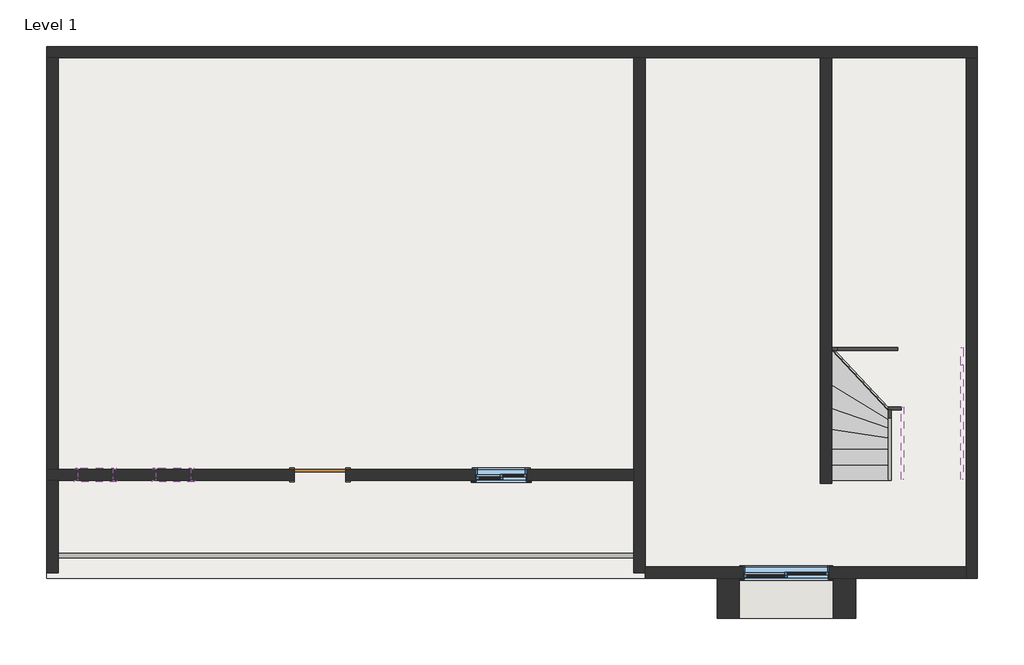
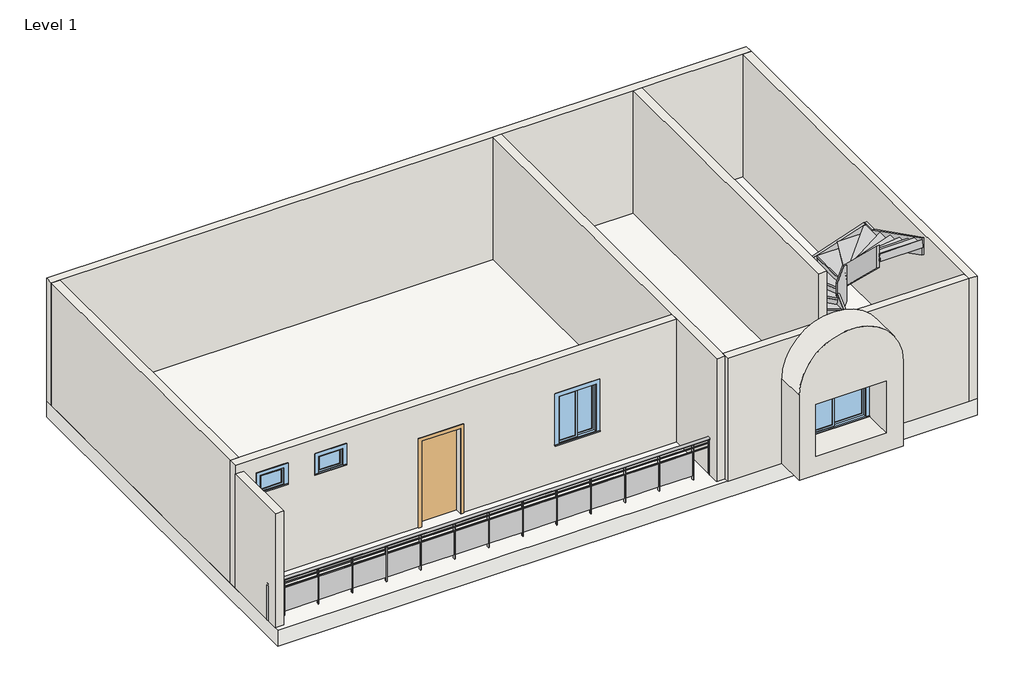
# One storey, incomplete: 9 walls, 8 members, 4 windows, 1 door, 1 railing, 1 slab, 1 stair flight.
"""IFC4 building model written with IfcOpenShell, lengths in millimetres."""

from ifc_helpers import new_model, si_unit, point, frame, origin, place, context, project, spatial, polyline, ellipse_curve, trimmed, outline, extrude, faceted_brep, transform, mapped, element, save
from ifc_brep_helpers import plane_surface, extruded_surface, advanced_brep
from components import m_single_flush_0915_x_2134mm_6a9e8738, stair_flight_50mm_tread_25mm_nosing_13mm_riser_620a4597, walls_3_walls_3_3787e265, window_242facca, window_c4d7a2b1, window_372a270f

model = new_model("IFC4")

# Units and contexts
model_context = context("Model", 3, world=origin())
ifc_project = project(units=[si_unit("LENGTHUNIT", "METRE", prefix="MILLI")], contexts=[model_context])

# Site, building, storey
site = spatial("IfcSite", under=ifc_project)
building = spatial("IfcBuilding", under=site)
storey = spatial("IfcBuildingStorey", under=building, Name="Level 1", Elevation=3048.0)

# Door
placement = place(None, origin())
m_single_flush_0915_x_2134mm_shape = m_single_flush_0915_x_2134mm_6a9e8738(model_context)
element("IfcDoor", 1, ObjectType="M_Single-Flush : 0915 x 2134mm", at=placement, inside=storey, context=model_context, shape_type="MappedRepresentation", body=[
    mapped(m_single_flush_0915_x_2134mm_shape, transform((255.2261575, -1309.9510925, 3048.0), x_axis=(1.0, 0.0, 0.0), y_axis=(0.0, 1.0, 0.0), z_axis=(0.0, 0.0, 1.0))),
])

# Members
element("IfcMember", 2, ObjectType="Stringer - 50mm Width", at=placement, inside=storey, context=model_context, shape_type="SweptSolid", body=[
    extrude(outline(polyline([(-1405.5848061, 3048.0), (-1405.5848061, 3306.6349517), (889.7143644, 4326.8592385), (889.7143644, 3889.1257613), (-1002.6491944, 3048.0), (-1405.5848061, 3048.0)])), frame((9239.7239729, 0.0, 0.0), z_axis=(1.0, 0.0, 0.0), x_axis=(0.0, 1.0, 0.0)), (0.0, 0.0, 1.0), 50.0),
])
element("IfcMember", 3, ObjectType="Stringer - 50mm Width", at=placement, inside=storey, context=model_context, shape_type="SweptSolid", body=[
    extrude(outline(polyline([(9239.7239729, 889.7143644), (9239.7239729, 939.7143644), (9388.2243256, 939.7143644), (9388.2243256, 889.7143644), (9239.7239729, 889.7143644)])), frame((0.0, 0.0, 3889.1257613), z_axis=(0.0, 0.0, 1.0), x_axis=(1.0, 0.0, 0.0)), (0.0, 0.0, 1.0), 437.7334772),
])
element("IfcMember", 4, ObjectType="Stringer - 50mm Width", at=placement, inside=storey, context=model_context, shape_type="SweptSolid", body=[
    extrude(outline(polyline([(4326.8592385, 9388.2243256), (3889.1257613, 9388.2243256), (4620.7976317, 11564.7755354), (5053.604341, 11564.7755354), (5053.604341, 11550.1195633), (4326.8592385, 9388.2243256)])), frame((0.0, 889.7143644, 0.0), z_axis=(0.0, 1.0, 0.0), x_axis=(0.0, 0.0, 1.0)), (0.0, 0.0, 1.0), 50.0),
])
element("IfcMember", 5, ObjectType="Stringer - 50mm Width", at=placement, inside=storey, context=model_context, shape_type="SweptSolid", body=[
    extrude(outline(polyline([(11564.7755354, 939.7143644), (11614.7755354, 939.7143644), (11614.7755354, 631.1318326), (11564.7755354, 631.1318326), (11564.7755354, 939.7143644)])), frame((0.0, 0.0, 4631.6082668), z_axis=(0.0, 0.0, 1.0), x_axis=(1.0, 0.0, 0.0)), (0.0, 0.0, 1.0), 421.9960743),
])
element("IfcMember", 6, ObjectType="Stringer - 50mm Width", at=placement, inside=storey, context=model_context, shape_type="SweptSolid", body=[
    extrude(outline(polyline([(631.1318326, 5053.604341), (631.1318326, 4631.6082668), (-1386.5243932, 5651.0031346), (-1386.5243932, 6072.9992088), (631.1318326, 5053.604341)])), frame((11564.7755354, 0.0, 0.0), z_axis=(1.0, 0.0, 0.0), x_axis=(0.0, 1.0, 0.0)), (0.0, 0.0, 1.0), 50.0),
])
element("IfcMember", 7, ObjectType="Stringer - 50mm Width", at=placement, inside=storey, context=model_context, shape_type="SweptSolid", body=[
    extrude(outline(polyline([(-1405.5848061, 3048.0), (-1405.5848061, 3215.9450175), (-160.3114169, 4397.3254446), (-160.3114169, 3845.9612039), (-1001.4290028, 3048.0), (-1405.5848061, 3048.0)])), frame((10289.7497541, 0.0, 0.0), z_axis=(1.0, 0.0, 0.0), x_axis=(0.0, 1.0, 0.0)), (0.0, 0.0, 1.0), 50.0),
])
element("IfcMember", 8, ObjectType="Stringer - 50mm Width", at=placement, inside=storey, context=model_context, shape_type="SweptSolid", body=[
    extrude(outline(polyline([(4651.1179686, 10289.7497541), (3893.3957848, 10289.7497541), (3893.3957848, 10414.0648587), (4141.6297966, 10514.7497541), (5030.7346373, 10514.7497541), (5030.7346373, 10443.7240799), (4651.1179686, 10289.7497541)])), frame((0.0, -160.3114169, 0.0), z_axis=(0.0, 1.0, 0.0), x_axis=(0.0, 0.0, 1.0)), (0.0, 0.0, 1.0), 50.0),
])
element("IfcMember", 9, ObjectType="Stringer - 50mm Width", at=placement, inside=storey, context=model_context, shape_type="SweptSolid", body=[
    extrude(outline(polyline([(-110.3114169, 5030.7346373), (-110.3114169, 4477.3598105), (-1386.5243932, 5697.3941307), (-1386.5243932, 6250.7689575), (-110.3114169, 5030.7346373)])), frame((10514.7497541, 0.0, 0.0), z_axis=(1.0, 0.0, 0.0), x_axis=(0.0, 1.0, 0.0)), (0.0, 0.0, 1.0), 50.0),
])

# Railing
element("IfcRailing", 10, ObjectType="Glass Panel - Bottom Fill", at=placement, inside=storey, context=model_context, shape_type="SolidModel", body=[
    advanced_brep(
    [(-4569.1738425, -2694.5603274, 3948.0), (-4569.1738425, -2774.5603274, 3948.0), (5794.0261575, -2694.5603274, 3948.0), (5794.0261575, -2774.5603274, 3948.0)],
    [
        (0, 1, ellipse_curve(frame((-4569.1738425, -2734.5603274, 3948.0), z_axis=(-1.0, 0.0, 0.0), x_axis=(0.0, -1.0, 0.0)), 40.0, 30.0)),
        (1, 0, ellipse_curve(frame((-4569.1738425, -2734.5603274, 3948.0), z_axis=(-1.0, 0.0, 0.0), x_axis=(0.0, -1.0, 0.0)), 40.0, 30.0)),
        (2, 3, ellipse_curve(frame((5794.0261575, -2734.5603274, 3948.0), z_axis=(1.0, 0.0, 0.0), x_axis=(0.0, -1.0, 0.0)), 40.0, 30.0)),
        (3, 2, ellipse_curve(frame((5794.0261575, -2734.5603274, 3948.0), z_axis=(1.0, 0.0, 0.0), x_axis=(0.0, -1.0, 0.0)), 40.0, 30.0)),
        (1, 3),
        (2, 0),
    ],
    [
        plane_surface(frame((-4569.1738425, -2734.5603274, 3948.0), z_axis=(-1.0, 0.0, 0.0), x_axis=(0.0, 1.0, 0.0))),
        plane_surface(frame((5794.0261575, -2734.5603274, 3948.0), z_axis=(1.0, 0.0, 0.0), x_axis=(0.0, 1.0, 0.0))),
        extruded_surface(trimmed(ellipse_curve(frame((5794.0261575, -2734.5603274, 3948.0), z_axis=(-1.0, 0.0, 0.0), x_axis=(0.0, -1.0, 0.0)), 40.0, 30.0), [point((5794.0261575, -2774.5603274, 3948.0))], [point((5794.0261575, -2694.5603274, 3948.0))], True, "CARTESIAN"), (-10363.2, 0.0, 0.0), 10363.2),
        extruded_surface(trimmed(ellipse_curve(frame((5794.0261575, -2734.5603274, 3948.0), z_axis=(-1.0, 0.0, 0.0), x_axis=(0.0, -1.0, 0.0)), 40.0, 30.0), [point((5794.0261575, -2694.5603274, 3948.0))], [point((5794.0261575, -2774.5603274, 3948.0))], True, "CARTESIAN"), (-10363.2, 0.0, 0.0), 10363.2),
    ],
    [
        (0, [[1, 2]]),
        (1, [[3, 4]]),
        (2, [[-2, 5, -3, 6]]),
        (3, [[-1, -6, -4, -5]]),
    ],
),
    extrude(outline(polyline([(-4569.1738425, -2743.9510925), (-4569.1738425, -2723.9510925), (5794.0261575, -2723.9510925), (5794.0261575, -2743.9510925), (-4569.1738425, -2743.9510925)])), frame((0.0, 0.0, 3828.0), z_axis=(0.0, 0.0, 1.0), x_axis=(1.0, 0.0, 0.0)), (0.0, 0.0, 1.0), 20.0),
    extrude(outline(polyline([(-4569.1738425, -2743.9510925), (-4569.1738425, -2723.9510925), (5794.0261575, -2723.9510925), (5794.0261575, -2743.9510925), (-4569.1738425, -2743.9510925)])), frame((0.0, 0.0, 3728.0), z_axis=(0.0, 0.0, 1.0), x_axis=(1.0, 0.0, 0.0)), (0.0, 0.0, 1.0), 20.0),
    extrude(outline(polyline([(5406.4261575, -2708.9510925), (5418.4261575, -2708.9510925), (5418.4261575, -2758.9510925), (5406.4261575, -2758.9510925), (5406.4261575, -2708.9510925)])), frame((0.0, 0.0, 3048.0), z_axis=(0.0, 0.0, 1.0), x_axis=(1.0, 0.0, 0.0)), (0.0, 0.0, 1.0), 869.8465326),
    extrude(outline(polyline([(4612.4261575, -2735.6759026), (5412.4261575, -2735.6759026), (5412.4261575, -2740.6759026), (4612.4261575, -2740.6759026), (4612.4261575, -2735.6759026)])), frame((0.0, 0.0, 3148.0), z_axis=(0.0, 0.0, 1.0), x_axis=(1.0, 0.0, 0.0)), (0.0, 0.0, 1.0), 580.0),
    extrude(outline(polyline([(4606.4261575, -2708.9510925), (4618.4261575, -2708.9510925), (4618.4261575, -2758.9510925), (4606.4261575, -2758.9510925), (4606.4261575, -2708.9510925)])), frame((0.0, 0.0, 3048.0), z_axis=(0.0, 0.0, 1.0), x_axis=(1.0, 0.0, 0.0)), (0.0, 0.0, 1.0), 869.8465326),
    extrude(outline(polyline([(3812.4261575, -2735.6759026), (4612.4261575, -2735.6759026), (4612.4261575, -2740.6759026), (3812.4261575, -2740.6759026), (3812.4261575, -2735.6759026)])), frame((0.0, 0.0, 3148.0), z_axis=(0.0, 0.0, 1.0), x_axis=(1.0, 0.0, 0.0)), (0.0, 0.0, 1.0), 580.0),
    extrude(outline(polyline([(3806.4261575, -2708.9510925), (3818.4261575, -2708.9510925), (3818.4261575, -2758.9510925), (3806.4261575, -2758.9510925), (3806.4261575, -2708.9510925)])), frame((0.0, 0.0, 3048.0), z_axis=(0.0, 0.0, 1.0), x_axis=(1.0, 0.0, 0.0)), (0.0, 0.0, 1.0), 869.8465326),
    extrude(outline(polyline([(3012.4261575, -2735.6759026), (3812.4261575, -2735.6759026), (3812.4261575, -2740.6759026), (3012.4261575, -2740.6759026), (3012.4261575, -2735.6759026)])), frame((0.0, 0.0, 3148.0), z_axis=(0.0, 0.0, 1.0), x_axis=(1.0, 0.0, 0.0)), (0.0, 0.0, 1.0), 580.0),
    extrude(outline(polyline([(3006.4261575, -2708.9510925), (3018.4261575, -2708.9510925), (3018.4261575, -2758.9510925), (3006.4261575, -2758.9510925), (3006.4261575, -2708.9510925)])), frame((0.0, 0.0, 3048.0), z_axis=(0.0, 0.0, 1.0), x_axis=(1.0, 0.0, 0.0)), (0.0, 0.0, 1.0), 869.8465326),
    extrude(outline(polyline([(2212.4261575, -2735.6759026), (3012.4261575, -2735.6759026), (3012.4261575, -2740.6759026), (2212.4261575, -2740.6759026), (2212.4261575, -2735.6759026)])), frame((0.0, 0.0, 3148.0), z_axis=(0.0, 0.0, 1.0), x_axis=(1.0, 0.0, 0.0)), (0.0, 0.0, 1.0), 580.0),
    extrude(outline(polyline([(2206.4261575, -2708.9510925), (2218.4261575, -2708.9510925), (2218.4261575, -2758.9510925), (2206.4261575, -2758.9510925), (2206.4261575, -2708.9510925)])), frame((0.0, 0.0, 3048.0), z_axis=(0.0, 0.0, 1.0), x_axis=(1.0, 0.0, 0.0)), (0.0, 0.0, 1.0), 869.8465326),
    extrude(outline(polyline([(1412.4261575, -2735.6759026), (2212.4261575, -2735.6759026), (2212.4261575, -2740.6759026), (1412.4261575, -2740.6759026), (1412.4261575, -2735.6759026)])), frame((0.0, 0.0, 3148.0), z_axis=(0.0, 0.0, 1.0), x_axis=(1.0, 0.0, 0.0)), (0.0, 0.0, 1.0), 580.0),
    extrude(outline(polyline([(1406.4261575, -2708.9510925), (1418.4261575, -2708.9510925), (1418.4261575, -2758.9510925), (1406.4261575, -2758.9510925), (1406.4261575, -2708.9510925)])), frame((0.0, 0.0, 3048.0), z_axis=(0.0, 0.0, 1.0), x_axis=(1.0, 0.0, 0.0)), (0.0, 0.0, 1.0), 869.8465326),
    extrude(outline(polyline([(612.4261575, -2735.6759026), (1412.4261575, -2735.6759026), (1412.4261575, -2740.6759026), (612.4261575, -2740.6759026), (612.4261575, -2735.6759026)])), frame((0.0, 0.0, 3148.0), z_axis=(0.0, 0.0, 1.0), x_axis=(1.0, 0.0, 0.0)), (0.0, 0.0, 1.0), 580.0),
    extrude(outline(polyline([(606.4261575, -2708.9510925), (618.4261575, -2708.9510925), (618.4261575, -2758.9510925), (606.4261575, -2758.9510925), (606.4261575, -2708.9510925)])), frame((0.0, 0.0, 3048.0), z_axis=(0.0, 0.0, 1.0), x_axis=(1.0, 0.0, 0.0)), (0.0, 0.0, 1.0), 869.8465326),
    extrude(outline(polyline([(-187.5738425, -2735.6759026), (612.4261575, -2735.6759026), (612.4261575, -2740.6759026), (-187.5738425, -2740.6759026), (-187.5738425, -2735.6759026)])), frame((0.0, 0.0, 3148.0), z_axis=(0.0, 0.0, 1.0), x_axis=(1.0, 0.0, 0.0)), (0.0, 0.0, 1.0), 580.0),
    extrude(outline(polyline([(-193.5738425, -2708.9510925), (-181.5738425, -2708.9510925), (-181.5738425, -2758.9510925), (-193.5738425, -2758.9510925), (-193.5738425, -2708.9510925)])), frame((0.0, 0.0, 3048.0), z_axis=(0.0, 0.0, 1.0), x_axis=(1.0, 0.0, 0.0)), (0.0, 0.0, 1.0), 869.8465326),
    extrude(outline(polyline([(-987.5738425, -2735.6759026), (-187.5738425, -2735.6759026), (-187.5738425, -2740.6759026), (-987.5738425, -2740.6759026), (-987.5738425, -2735.6759026)])), frame((0.0, 0.0, 3148.0), z_axis=(0.0, 0.0, 1.0), x_axis=(1.0, 0.0, 0.0)), (0.0, 0.0, 1.0), 580.0),
    extrude(outline(polyline([(-993.5738425, -2708.9510925), (-981.5738425, -2708.9510925), (-981.5738425, -2758.9510925), (-993.5738425, -2758.9510925), (-993.5738425, -2708.9510925)])), frame((0.0, 0.0, 3048.0), z_axis=(0.0, 0.0, 1.0), x_axis=(1.0, 0.0, 0.0)), (0.0, 0.0, 1.0), 869.8465326),
    extrude(outline(polyline([(-1787.5738425, -2735.6759026), (-987.5738425, -2735.6759026), (-987.5738425, -2740.6759026), (-1787.5738425, -2740.6759026), (-1787.5738425, -2735.6759026)])), frame((0.0, 0.0, 3148.0), z_axis=(0.0, 0.0, 1.0), x_axis=(1.0, 0.0, 0.0)), (0.0, 0.0, 1.0), 580.0),
    extrude(outline(polyline([(-1793.5738425, -2708.9510925), (-1781.5738425, -2708.9510925), (-1781.5738425, -2758.9510925), (-1793.5738425, -2758.9510925), (-1793.5738425, -2708.9510925)])), frame((0.0, 0.0, 3048.0), z_axis=(0.0, 0.0, 1.0), x_axis=(1.0, 0.0, 0.0)), (0.0, 0.0, 1.0), 869.8465326),
    extrude(outline(polyline([(-2587.5738425, -2735.6759026), (-1787.5738425, -2735.6759026), (-1787.5738425, -2740.6759026), (-2587.5738425, -2740.6759026), (-2587.5738425, -2735.6759026)])), frame((0.0, 0.0, 3148.0), z_axis=(0.0, 0.0, 1.0), x_axis=(1.0, 0.0, 0.0)), (0.0, 0.0, 1.0), 580.0),
    extrude(outline(polyline([(-2593.5738425, -2708.9510925), (-2581.5738425, -2708.9510925), (-2581.5738425, -2758.9510925), (-2593.5738425, -2758.9510925), (-2593.5738425, -2708.9510925)])), frame((0.0, 0.0, 3048.0), z_axis=(0.0, 0.0, 1.0), x_axis=(1.0, 0.0, 0.0)), (0.0, 0.0, 1.0), 869.8465326),
    extrude(outline(polyline([(-3387.5738425, -2735.6759026), (-2587.5738425, -2735.6759026), (-2587.5738425, -2740.6759026), (-3387.5738425, -2740.6759026), (-3387.5738425, -2735.6759026)])), frame((0.0, 0.0, 3148.0), z_axis=(0.0, 0.0, 1.0), x_axis=(1.0, 0.0, 0.0)), (0.0, 0.0, 1.0), 580.0),
    extrude(outline(polyline([(-3393.5738425, -2708.9510925), (-3381.5738425, -2708.9510925), (-3381.5738425, -2758.9510925), (-3393.5738425, -2758.9510925), (-3393.5738425, -2708.9510925)])), frame((0.0, 0.0, 3048.0), z_axis=(0.0, 0.0, 1.0), x_axis=(1.0, 0.0, 0.0)), (0.0, 0.0, 1.0), 869.8465326),
    extrude(outline(polyline([(-4187.5738425, -2735.6759026), (-3387.5738425, -2735.6759026), (-3387.5738425, -2740.6759026), (-4187.5738425, -2740.6759026), (-4187.5738425, -2735.6759026)])), frame((0.0, 0.0, 3148.0), z_axis=(0.0, 0.0, 1.0), x_axis=(1.0, 0.0, 0.0)), (0.0, 0.0, 1.0), 580.0),
    extrude(outline(polyline([(-4193.5738425, -2708.9510925), (-4181.5738425, -2708.9510925), (-4181.5738425, -2758.9510925), (-4193.5738425, -2758.9510925), (-4193.5738425, -2708.9510925)])), frame((0.0, 0.0, 3048.0), z_axis=(0.0, 0.0, 1.0), x_axis=(1.0, 0.0, 0.0)), (0.0, 0.0, 1.0), 869.8465326),
    extrude(outline(polyline([(5786.0261575, -2708.9510925), (5798.0261575, -2708.9510925), (5798.0261575, -2758.9510925), (5786.0261575, -2758.9510925), (5786.0261575, -2708.9510925)])), frame((0.0, 0.0, 3048.0), z_axis=(0.0, 0.0, 1.0), x_axis=(1.0, 0.0, 0.0)), (0.0, 0.0, 1.0), 869.8465326),
    extrude(outline(polyline([(-4573.1738425, -2708.9510925), (-4561.1738425, -2708.9510925), (-4561.1738425, -2758.9510925), (-4573.1738425, -2758.9510925), (-4573.1738425, -2708.9510925)])), frame((0.0, 0.0, 3048.0), z_axis=(0.0, 0.0, 1.0), x_axis=(1.0, 0.0, 0.0)), (0.0, 0.0, 1.0), 869.8465326),
])

# Slab
element("IfcSlab", 11, ObjectType="Generic Floor - 400mm", at=placement, inside=storey, context=model_context, shape_type="SweptSolid", body=[
    extrude(outline(polyline([(11861.7023789, 6257.6489075), (11861.7023789, -3138.7510925), (-4569.1738425, -3138.7510925), (-4569.1738425, 6257.6489075), (11861.7023789, 6257.6489075)])), frame((0.0, 0.0, 2648.0), z_axis=(0.0, 0.0, 1.0), x_axis=(1.0, 0.0, 0.0)), (0.0, 0.0, 1.0), 400.0),
])

# Stair flight
stair_flight_50mm_tread_25mm_nosing_13mm_riser_shape = stair_flight_50mm_tread_25mm_nosing_13mm_riser_620a4597(model_context)
element("IfcStairFlight", 12, ObjectType="50mm Tread 25mm Nosing 13mm Riser", at=placement, inside=storey, context=model_context, shape_type="MappedRepresentation", body=[
    mapped(stair_flight_50mm_tread_25mm_nosing_13mm_riser_shape, transform((0.0, 0.0, 0.0), x_axis=(1.0, 0.0, 0.0), y_axis=(0.0, 1.0, 0.0), z_axis=(0.0, 0.0, 1.0))),
])

# Walls
element("IfcWall", 13, ObjectType="Generic - 9\"", at=placement, inside=storey, context=model_context, shape_type="Brep", body=[
    faceted_brep([(-4569.1738425, 6057.6489075, 3048.0), (-4369.1738425, 6057.6489075, 3048.0), (5794.0261575, 6057.6489075, 3048.0), (5994.0261575, 6057.6489075, 3048.0), (9086.6508164, 6057.6489075, 3048.0), (9286.6508164, 6057.6489075, 3048.0), (11661.7023789, 6057.6489075, 3048.0), (11861.7023789, 6057.6489075, 3048.0), (11861.7023789, 6057.6489075, 6096.0), (11661.7023789, 6057.6489075, 6096.0), (9286.6508164, 6057.6489075, 6096.0), (9086.6508164, 6057.6489075, 6096.0), (5994.0261575, 6057.6489075, 6096.0), (5794.0261575, 6057.6489075, 6096.0), (-4369.1738425, 6057.6489075, 6096.0), (-4569.1738425, 6057.6489075, 6096.0), (-4569.1738425, 6257.6489075, 3048.0), (-4569.1738425, 6257.6489075, 6096.0), (11861.7023789, 6257.6489075, 6096.0), (11861.7023789, 6257.6489075, 3048.0)], [[[0, 1, 2, 3, 4, 5, 6, 7, 8, 9, 10, 11, 12, 13, 14, 15]], [[16, 17, 18, 19]], [[7, 6, 5, 4, 3, 2, 1, 0, 16, 19]], [[15, 14, 13, 12, 11, 10, 9, 8, 18, 17]], [[0, 15, 17, 16]], [[8, 7, 19, 18]]]),
])
element("IfcWall", 14, ObjectType="Generic - 9\"", at=placement, inside=storey, context=model_context, shape_type="SweptSolid", body=[
    extrude(outline(polyline([(-4569.1738425, -1209.9510925), (-4569.1738425, 6057.6489075), (-4369.1738425, 6057.6489075), (-4369.1738425, -1209.9510925), (-4569.1738425, -1209.9510925)])), frame((0.0, 0.0, 3048.0), z_axis=(0.0, 0.0, 1.0), x_axis=(1.0, 0.0, 0.0)), (0.0, 0.0, 1.0), 3048.0),
])
element("IfcWall", 15, ObjectType="Generic - 9\"", at=placement, inside=storey, context=model_context, shape_type="Brep", body=[
    faceted_brep([(712.7261575, -1409.9510925, 5182.0), (712.7261575, -1409.9510925, 3048.0), (5794.0261575, -1409.9510925, 3048.0), (5794.0261575, -1409.9510925, 6096.0), (-4569.1738425, -1409.9510925, 6096.0), (-4569.1738425, -1409.9510925, 5877.7029463), (-4569.1738425, -1409.9510925, 3048.0), (-4369.1738425, -1409.9510925, 3048.0), (-202.2738425, -1409.9510925, 3048.0), (-202.2738425, -1409.9510925, 5182.0), (2998.4261575, -1409.9510925, 5181.6), (3912.8261575, -1409.9510925, 5181.6), (3912.8261575, -1409.9510925, 3962.4), (2998.4261575, -1409.9510925, 3962.4), (-4011.9738425, -1409.9510925, 5664.2), (-3402.3738425, -1409.9510925, 5664.2), (-3402.3738425, -1409.9510925, 5207.0), (-4011.9738425, -1409.9510925, 5207.0), (-2640.3738425, -1409.9510925, 5664.2), (-2030.7738425, -1409.9510925, 5664.2), (-2030.7738425, -1409.9510925, 5207.0), (-2640.3738425, -1409.9510925, 5207.0), (5794.0261575, -1209.9510925, 3048.0), (712.7261575, -1209.9510925, 3048.0), (712.7261575, -1209.9510925, 5182.0), (-202.2738425, -1209.9510925, 5182.0), (-202.2738425, -1209.9510925, 3048.0), (-4369.1738425, -1209.9510925, 3048.0), (-4569.1738425, -1209.9510925, 3048.0), (-4569.1738425, -1209.9510925, 6096.0), (-4369.1738425, -1209.9510925, 6096.0), (5794.0261575, -1209.9510925, 6096.0), (2998.4261575, -1209.9510925, 5181.6), (2998.4261575, -1209.9510925, 3962.4), (3912.8261575, -1209.9510925, 3962.4), (3912.8261575, -1209.9510925, 5181.6), (-4011.9738425, -1209.9510925, 5664.2), (-4011.9738425, -1209.9510925, 5207.0), (-3402.3738425, -1209.9510925, 5207.0), (-3402.3738425, -1209.9510925, 5664.2), (-2640.3738425, -1209.9510925, 5664.2), (-2640.3738425, -1209.9510925, 5207.0), (-2030.7738425, -1209.9510925, 5207.0), (-2030.7738425, -1209.9510925, 5664.2)], [[[0, 1, 2, 3, 4, 5, 6, 7, 8, 9], [10, 11, 12, 13], [14, 15, 16, 17], [18, 19, 20, 21]], [[22, 23, 24, 25, 26, 27, 28, 29, 30, 31], [32, 33, 34, 35], [36, 37, 38, 39], [40, 41, 42, 43]], [[3, 2, 22, 31]], [[24, 23, 1, 0]], [[25, 24, 0, 9]], [[26, 25, 9, 8]], [[33, 32, 10, 13]], [[34, 33, 13, 12]], [[35, 34, 12, 11]], [[32, 35, 11, 10]], [[4, 29, 28, 6, 5]], [[37, 36, 14, 17]], [[38, 37, 17, 16]], [[39, 38, 16, 15]], [[36, 39, 15, 14]], [[41, 40, 18, 21]], [[42, 41, 21, 20]], [[43, 42, 20, 19]], [[40, 43, 19, 18]], [[2, 1, 23, 22]], [[8, 7, 6, 28, 27, 26]], [[4, 3, 31, 30, 29]]]),
])
element("IfcWall", 16, ObjectType="Generic - 9\"", at=placement, inside=storey, context=model_context, shape_type="Brep", body=[
    faceted_brep([(11861.7023789, -3138.7510925, 3048.0), (11861.7023789, 6057.6489075, 3048.0), (11861.7023789, 6057.6489075, 6096.0), (11861.7023789, -3138.7510925, 6096.0), (11661.7023789, -3138.7510925, 3048.0), (11661.7023789, -3138.7510925, 6096.0), (11661.7023789, -2938.7510925, 6096.0), (11661.7023789, 6057.6489075, 6096.0), (11661.7023789, 6057.6489075, 3048.0), (11661.7023789, -2938.7510925, 3048.0)], [[[0, 1, 2, 3]], [[4, 5, 6, 7, 8, 9]], [[1, 0, 4, 9, 8]], [[3, 2, 7, 6, 5]], [[2, 1, 8, 7]], [[0, 3, 5, 4]]]),
])
element("IfcWall", 17, ObjectType="Generic - 9\"", at=placement, inside=storey, context=model_context, shape_type="Brep", body=[
    faceted_brep([(5794.0261575, 6057.6489075, 3048.0), (5794.0261575, -1209.9510925, 3048.0), (5794.0261575, -1409.9510925, 3048.0), (5794.0261575, -3038.7510925, 3048.0), (5794.0261575, -3038.7510925, 6096.0), (5794.0261575, -1409.9510925, 6096.0), (5794.0261575, -1209.9510925, 6096.0), (5794.0261575, 6057.6489075, 6096.0), (5994.0261575, 6057.6489075, 3048.0), (5994.0261575, 6057.6489075, 6096.0), (5994.0261575, -2938.7510925, 6096.0), (5994.0261575, -3038.7510925, 6096.0), (5994.0261575, -3038.7510925, 3048.0), (5994.0261575, -2938.7510925, 3048.0)], [[[0, 1, 2, 3, 4, 5, 6, 7]], [[8, 9, 10, 11, 12, 13]], [[3, 2, 1, 0, 8, 13, 12]], [[4, 3, 12, 11]], [[7, 6, 5, 4, 11, 10, 9]], [[0, 7, 9, 8]]]),
])
element("IfcWall", 18, ObjectType="Generic - 9\"", at=placement, inside=storey, context=model_context, shape_type="Brep", body=[
    faceted_brep([(11661.7023789, -2938.7510925, 3048.0), (5994.0261575, -2938.7510925, 3048.0), (5994.0261575, -2938.7510925, 6096.0), (11661.7023789, -2938.7510925, 6096.0), (7722.8261575, -2938.7510925, 4730.6578847), (7722.8261575, -2938.7510925, 3511.4578847), (9246.8261575, -2938.7510925, 3511.4578847), (9246.8261575, -2938.7510925, 4730.6578847), (11661.7023789, -3138.7510925, 3048.0), (11661.7023789, -3138.7510925, 6096.0), (5994.0261575, -3138.7510925, 6096.0), (5994.0261575, -3138.7510925, 3048.0), (7722.8261575, -3138.7510925, 4730.6578847), (9246.8261575, -3138.7510925, 4730.6578847), (9246.8261575, -3138.7510925, 3511.4578847), (7722.8261575, -3138.7510925, 3511.4578847), (5994.0261575, -3038.7510925, 3048.0), (5994.0261575, -3038.7510925, 6096.0)], [[[0, 1, 2, 3], [4, 5, 6, 7]], [[8, 9, 10, 11], [12, 13, 14, 15]], [[1, 0, 8, 11, 16]], [[3, 2, 17, 10, 9]], [[2, 1, 16, 11, 10, 17]], [[0, 3, 9, 8]], [[5, 4, 12, 15]], [[6, 5, 15, 14]], [[7, 6, 14, 13]], [[4, 7, 13, 12]]]),
])
element("IfcWall", 19, ObjectType="Generic - 9\"", at=placement, inside=storey, context=model_context, shape_type="SweptSolid", body=[
    extrude(outline(polyline([(9086.6508164, -1462.3510925), (9086.6508164, 6057.6489075), (9286.6508164, 6057.6489075), (9286.6508164, -1462.3510925), (9086.6508164, -1462.3510925)])), frame((0.0, 0.0, 3048.0), z_axis=(0.0, 0.0, 1.0), x_axis=(1.0, 0.0, 0.0)), (0.0, 0.0, 1.0), 3048.0),
])
element("IfcWall", 20, ObjectType="Generic - 9\"", at=placement, inside=storey, context=model_context, shape_type="SweptSolid", body=[
    extrude(outline(polyline([(-4569.1738425, -3038.7510925), (-4569.1738425, -1409.9510925), (-4369.1738425, -1409.9510925), (-4369.1738425, -3038.7510925), (-4569.1738425, -3038.7510925)])), frame((0.0, 0.0, 3048.0), z_axis=(0.0, 0.0, 1.0), x_axis=(1.0, 0.0, 0.0)), (0.0, 0.0, 1.0), 2829.7029463),
])
walls_3_walls_3_shape = walls_3_walls_3_3787e265(model_context)
element("IfcWall", 21, ObjectType="Walls 3 : Walls 3", at=placement, inside=storey, context=model_context, shape_type="MappedRepresentation", body=[
    mapped(walls_3_walls_3_shape, transform((0.0, 0.0, 0.0), x_axis=(1.0, 0.0, 0.0), y_axis=(0.0, 1.0, 0.0), z_axis=(0.0, 0.0, 1.0))),
])

# Windows
window_shape = window_242facca(model_context)
element("IfcWindow", 22, ObjectType="Slider with Trim : 36\" x 48\"", at=placement, inside=storey, context=model_context, shape_type="MappedRepresentation", body=[
    mapped(window_shape, transform((3455.6261575, -1309.9510925, 3048.0), x_axis=(-1.0, 0.0, 0.0), y_axis=(0.0, -1.0, 0.0), z_axis=(0.0, 0.0, 1.0))),
])
window_2_shape = window_c4d7a2b1(model_context)
element("IfcWindow", 23, ObjectType="Slider with Trim : 60\" x 48\"", at=placement, inside=storey, context=model_context, shape_type="MappedRepresentation", body=[
    mapped(window_2_shape, transform((8484.8261575, -3038.7510925, 2597.0578847), x_axis=(-1.0, 0.0, 0.0), y_axis=(0.0, -1.0, 0.0), z_axis=(0.0, 0.0, 1.0))),
])
window_3_shape = window_372a270f(model_context)
element("IfcWindow", 24, ObjectType="Transom with Trim : 24\" x 18\"", at=placement, inside=storey, context=model_context, shape_type="MappedRepresentation", body=[
    mapped(window_3_shape, transform((-3745.2738425, -1309.9510925, 3048.0), x_axis=(-1.0, 0.0, 0.0), y_axis=(0.0, -1.0, 0.0), z_axis=(0.0, 0.0, 1.0))),
])
element("IfcWindow", 25, ObjectType="Transom with Trim : 24\" x 18\"", at=placement, inside=storey, context=model_context, shape_type="MappedRepresentation", body=[
    mapped(window_3_shape, transform((-2373.6738425, -1309.9510925, 3048.0), x_axis=(-1.0, 0.0, 0.0), y_axis=(0.0, -1.0, 0.0), z_axis=(0.0, 0.0, 1.0))),
])

save(model, "model.ifc")

# Revit data of these elements
# Type "M_Single-Flush : 0915 x 2134mm"
#   Type Mark = "15"
#   Thickness = 0' - 2.00787"
#   Height = 7' - 0.01575"
#   Trim Projection Ext = 0' - 0.98425"
#   Trim Projection Int = 0' - 0.98425"
#   Trim Width = 0' - 2.99213"
#   Width = 3' - 0.02362"
#   Door Material = Door - Panel
#   Frame Material = Door - Frame
#   Function = (empty or 0)
#   Wall Closure = (empty or 0)
# Type "Glass Panel - Bottom Fill"
#   built-in parameter 1008612 = 0.019685 (stored number, unit not read)
#   built-in parameter 1008611 = 0.019685 (stored number, unit not read)
#   built-in parameter 1008609 = 0.902231 (stored number, unit not read)
#   built-in parameter 1008604 = 0.19685 (stored number, unit not read)
#   built-in parameter 1008603 = 0.164042 (stored number, unit not read)
#   Railing Height = 2' - 11.43307"
#   built-in parameter 1008630 = 2
#   built-in parameter 1008610 = 2
# Type "Generic Floor - 400mm"
#   Function = 0
#   Layers, outside or top first: 1' - 3.74803" no material (function 1)
# Type "Generic - 9\""
#   Layers, outside or top first: 0' - 7.87402" no material (function 1)
# Type "Slider with Trim : 36\" x 48\""
#   Type Mark = "19"
#   Construction Type Id = "GSP4R"
#   Assembly Code = "B2020100"
#   Analytic Construction = "1/8 in Pilkington single glazing"
#   Visual Light Transmittance = 0.9
#   Solar Heat Gain Coefficient = 0.78
#   Heat Transfer Coefficient (U) = 3.6886 W/(m²·K)
#   Height = 4' - 0"
#   Default Sill Height = 3' - 0"
#   Trim Projection - Ext. = 0' - 0 3/4"
#   Trim Projection - Int. = 0' - 0 3/4"
#   Trim Width - Exterior = 0' - 3 1/2"
#   Trim Width - Interior = 0' - 3 1/2"
#   Width = 3' - 0"
#   Window Inset = 0' - 0 3/4"
#   Define Thermal Properties by = 1
#   Glass Pane Material = Glass
#   Sash Material = Sash
#   Trim Exterior Material = Trim
#   Trim Interior Material = Trim
#   Wall Closure = (empty or 0)
# Type "Slider with Trim : 60\" x 48\""
#   Type Mark = "22"
#   Construction Type Id = "GSP4R"
#   Assembly Code = "B2020100"
#   Analytic Construction = "1/8 in Pilkington single glazing"
#   Visual Light Transmittance = 0.9
#   Solar Heat Gain Coefficient = 0.78
#   Heat Transfer Coefficient (U) = 3.6886 W/(m²·K)
#   Height = 4' - 0"
#   Default Sill Height = 3' - 0"
#   Trim Projection - Ext. = 0' - 0 3/4"
#   Trim Projection - Int. = 0' - 0 3/4"
#   Trim Width - Exterior = 0' - 3 1/2"
#   Trim Width - Interior = 0' - 3 1/2"
#   Width = 5' - 0"
#   Window Inset = 0' - 0 3/4"
#   Define Thermal Properties by = 1
#   Glass Pane Material = Glass
#   Sash Material = Sash
#   Trim Exterior Material = Trim
#   Trim Interior Material = Trim
#   Wall Closure = (empty or 0)
# Type "Transom with Trim : 24\" x 18\""
#   Type Mark = "30"
#   Construction Type Id = "GSP4R"
#   Assembly Code = "B2020100"
#   Analytic Construction = "1/8 in Pilkington single glazing"
#   Visual Light Transmittance = 0.9
#   Solar Heat Gain Coefficient = 0.78
#   Heat Transfer Coefficient (U) = 3.6886 W/(m²·K)
#   Height = 1' - 6"
#   Default Sill Height = 7' - 1"
#   Trim Projection - Ext. = 0' - 0 1/2"
#   Trim Projection - Int. = 0' - 0 3/4"
#   Trim Width - Exterior = 0' - 3 1/2"
#   Trim Width - Interior = 0' - 3 1/2"
#   Width = 2' - 0"
#   Window Inset = 0' - 0 3/4"
#   Define Thermal Properties by = 1
#   Glass Pane Material = Glass
#   Sash Material = Sash
#   Trim Exterior Material = Trim
#   Trim Interior Material = Trim
#   Wall Closure = (empty or 0)
# Element 1 (IfcDoor, "M_Single-Flush : 0915 x 2134mm")
#   Phase Created = New Construction
#   Materials on its faces: "Door - Frame", "Door - Panel"
# Elements 2, 3, 4, 5, 6, 7, 8, 9 (IfcMember, "Stringer - 50mm Width")
#   Phase Created = New Construction
# Element 10 (IfcRailing, "Glass Panel - Bottom Fill")
#   Phase Created = New Construction
#   Materials on its faces: "Metal - Stainless Steel,Polished", "Glass"
# Element 11 (IfcSlab, "Generic Floor - 400mm")
#   Height Offset From Level = 0' - 0"
#   Phase Created = New Construction
#   Materials on its faces: "Default Roof"
# Element 12 (IfcStairFlight, "50mm Tread 25mm Nosing 13mm Riser")
#   Phase Created = New Construction
# Elements 13, 14, 15, 16, 17, 18, 19 (IfcWall, "Generic - 9\"")
#   Top Offset = 0' - 0"
#   Base Offset = 0' - 0"
#   Unconnected Height = 10' - 0"
#   wall height = 10' - 0"
#   Phase Created = New Construction
#   Base Constraint = Level 1
#   Materials on its faces: "Default Wall"
# Element 20 (IfcWall, "Generic - 9\"")
#   Top Offset = 0' - 0"
#   Base Offset = 0' - 0"
#   Unconnected Height = 9' - 3.40563"
#   wall height = 9' - 3.40563"
#   Phase Created = New Construction
#   Base Constraint = Level 1
#   Materials on its faces: "Default Wall"
# Element 21 (IfcWall, "Walls 3 : Walls 3")
#   Phase Created = New Construction
#   Materials on its faces: "Default Wall"
# Element 22 (IfcWindow, "Slider with Trim : 36\" x 48\"")
#   Mark = "7"
#   Phase Created = New Construction
#   Materials on its faces: "Sash", "Trim", "Glass"
# Element 23 (IfcWindow, "Slider with Trim : 60\" x 48\"")
#   Mark = "13"
#   Phase Created = New Construction
#   Materials on its faces: "Sash", "Trim", "Glass"
# Element 24 (IfcWindow, "Transom with Trim : 24\" x 18\"")
#   Mark = "10"
#   Phase Created = New Construction
#   Materials on its faces: "Sash", "Trim", "Glass"
# Element 25 (IfcWindow, "Transom with Trim : 24\" x 18\"")
#   Mark = "11"
#   Phase Created = New Construction
#   Materials on its faces: "Sash", "Trim", "Glass"
# Materials
#   "Door - Panel": class "Wood", colour RGB 114 82 51, transparency 0
#   "Door - Frame": colour RGB 153 76 43, transparency 0
#   "Glass": class "Glass", colour RGB 218 227 224, transparency 0.85, Description = "Soda Lime Glass", Cost = 0
#   "Sash": class "Wood", colour RGB 136 99 55, transparency 0
#   "Trim": class "Wood", colour RGB 224 178 126, transparency 0
#   "Metal - Stainless Steel,Polished": class "Metal", colour RGB 189 187 185, transparency 0, Cost = 0
#   "Default Roof": colour RGB 80 80 80, transparency 0
#   "Default Wall": colour RGB 80 80 80, transparency 0
